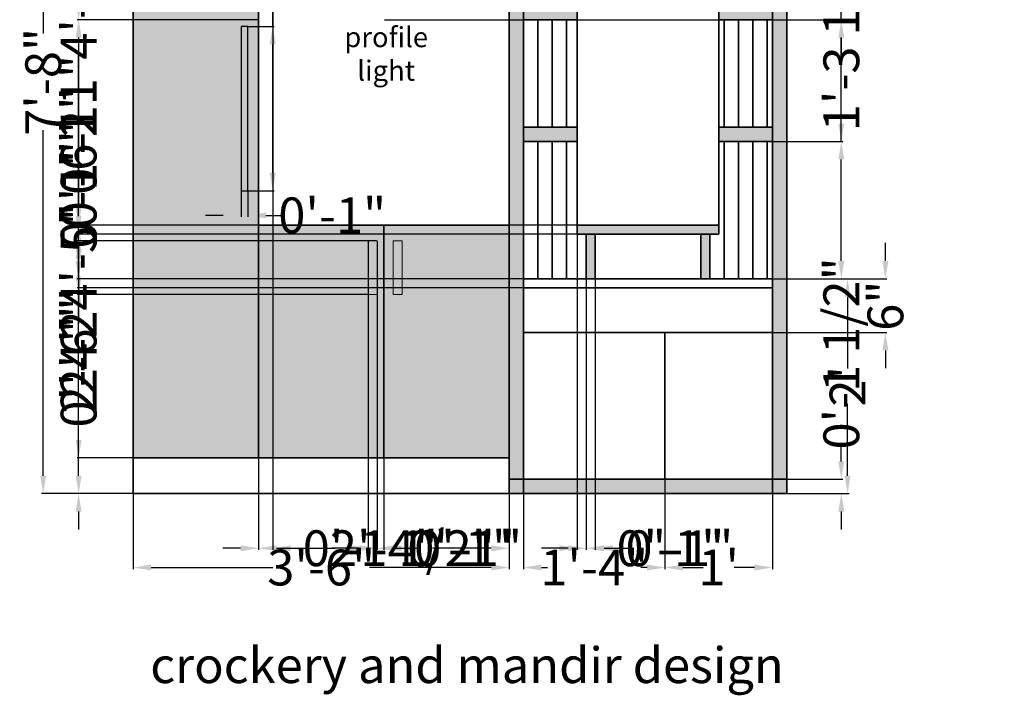
# Model space of a CAD drawing. Units: inches. Extents: x 15 to 125, y 28 to 155.
# Tile 1 of 2: x 15 to 125, y 28 to 104. Entities that reach past the tile are written whole.
import ezdxf

# ---------------------------------------------------------------- set-up
doc = ezdxf.new("R2010")
doc.units = ezdxf.units.IN
doc.header["$MEASUREMENT"] = 0
for name, color, linetype, lineweight in [('A-ANNO-DIMS', 2, 'Continuous', 18), ('A-ANNO-TEXT', 3, 'Continuous', 25), ('A-FURN', 7, 'Continuous', 35), ('A-FURN-HDWR', 8, 'Continuous', 18), ('A-FURN-PATT', 252, 'Continuous', 13)]:
    doc.layers.add(name, color=color, linetype=linetype, lineweight=lineweight)
doc.layers.add('Layer1', color=168, linetype='Continuous')
doc.styles.get("Standard").update_dxf_attribs({"font": 'arial.ttf'})
doc.dimstyles.get("Standard").update_dxf_attribs({"dimtxt": 4, "dimasz": 2, "dimexe": 0.18, "dimexo": 0.0625, "dimgap": 0.09, "dimtad": 0, "dimdec": 0, "dimzin": 0, "dimdsep": 46, "dimlunit": 4, "dimtxsty": 'Standard', "dimcen": 0.09, "dimadec": 0, "dimazin": 0, "dimtfac": 1, "dimtdec": 0, "dimtofl": 0, "dimtmove": 0, "dimatfit": 3, "dimfxl": 1, "dimtolj": 1, "dimtzin": 0, "dimarcsym": 0})

# ---------------------------------------------------------------- blocks, each defined once
blk = doc.blocks.new('*D1')
at = {"layer": 'A-ANNO-DIMS', "color": 0, "lineweight": -2, "transparency": 16777216}
for p, q in [((86.83, 52.41), (86.83, 42.44)), ((98.83, 52.41), (98.83, 42.44)), ((88.83, 42.62), (91.09, 42.62)), ((96.83, 42.62), (94.57, 42.62))]:
    blk.add_line(p, q, dxfattribs=at)
at = {"layer": 'A-ANNO-DIMS', "color": 0, "transparency": 16777216}
for points in [[(88.83, 42.95), (88.83, 42.29), (86.83, 42.62)], [(96.83, 42.95), (96.83, 42.29), (98.83, 42.62)]]:
    blk.add_solid(points, dxfattribs=at)
at = {"layer": 'Defpoints', "color": 0, "transparency": 16777216}
for p in [(86.83, 52.47), (98.83, 52.47), (98.83, 42.62)]:
    blk.add_point(p, dxfattribs=at)
at = {"layer": 'A-ANNO-DIMS', "color": 0, "transparency": 16777216, "insert": (92.83, 42.62), "char_height": 4, "attachment_point": 5}
blk.add_mtext("\\A1;1'", dxfattribs=at)
blk = doc.blocks.new('*D2')
at = {"layer": 'A-ANNO-DIMS', "color": 0, "lineweight": -2, "transparency": 16777216}
for p, q in [((71.03, 52.41), (71.03, 42.44)), ((86.83, 52.41), (86.83, 42.44)), ((73.03, 42.62), (73.71, 42.62)), ((84.83, 42.62), (84.15, 42.62))]:
    blk.add_line(p, q, dxfattribs=at)
at = {"layer": 'A-ANNO-DIMS', "color": 0, "transparency": 16777216}
for points in [[(73.03, 42.95), (73.03, 42.29), (71.03, 42.62)], [(84.83, 42.95), (84.83, 42.29), (86.83, 42.62)]]:
    blk.add_solid(points, dxfattribs=at)
at = {"layer": 'Defpoints', "color": 0, "transparency": 16777216}
for p in [(71.03, 52.47), (86.83, 52.47), (71.03, 42.62)]:
    blk.add_point(p, dxfattribs=at)
at = {"layer": 'A-ANNO-DIMS', "color": 0, "transparency": 16777216, "insert": (78.93, 42.62), "char_height": 4, "attachment_point": 5}
blk.add_mtext('\\A1;1\'-4"', dxfattribs=at)
blk = doc.blocks.new('*D3')
at = {"layer": 'A-ANNO-DIMS', "color": 0, "lineweight": -2, "transparency": 16777216}
for p, q in [((98.89, 74.87), (107.41, 74.87)), ((107.23, 72.87), (107.23, 64.84)), ((107.23, 52.87), (107.23, 60.91)), ((98.89, 50.87), (107.41, 50.87))]:
    blk.add_line(p, q, dxfattribs=at)
at = {"layer": 'A-ANNO-DIMS', "color": 0, "transparency": 16777216}
for points in [[(106.9, 72.87), (107.56, 72.87), (107.23, 74.87)], [(106.9, 52.87), (107.56, 52.87), (107.23, 50.87)]]:
    blk.add_solid(points, dxfattribs=at)
at = {"layer": 'Defpoints', "color": 0, "transparency": 16777216}
for p in [(98.83, 74.87), (107.23, 74.87), (98.83, 50.87)]:
    blk.add_point(p, dxfattribs=at)
at = {"layer": 'A-ANNO-DIMS', "color": 0, "transparency": 16777216, "insert": (107.23, 62.87), "char_height": 4, "attachment_point": 5, "rotation": 90}
blk.add_mtext("\\A1;2'", dxfattribs=at)
blk = doc.blocks.new('*D4')
at = {"layer": 'A-ANNO-DIMS', "color": 0, "lineweight": -2, "transparency": 16777216}
for p, q in [((111.45, 76.87), (111.45, 78.87)), ((98.89, 74.87), (111.63, 74.87)), ((98.89, 68.87), (111.63, 68.87)), ((111.45, 66.87), (111.45, 64.87))]:
    blk.add_line(p, q, dxfattribs=at)
at = {"layer": 'A-ANNO-DIMS', "color": 0, "transparency": 16777216}
for points in [[(111.12, 76.87), (111.79, 76.87), (111.45, 74.87)], [(111.12, 66.87), (111.79, 66.87), (111.45, 68.87)]]:
    blk.add_solid(points, dxfattribs=at)
at = {"layer": 'Defpoints', "color": 0, "transparency": 16777216}
for p in [(98.83, 74.87), (98.83, 68.87), (111.45, 68.87)]:
    blk.add_point(p, dxfattribs=at)
at = {"layer": 'A-ANNO-DIMS', "color": 0, "transparency": 16777216, "insert": (111.45, 71.87), "char_height": 4, "attachment_point": 5, "rotation": 90}
blk.add_mtext('\\A1;6"', dxfattribs=at)
blk = doc.blocks.new('*D8')
at = {"layer": 'A-ANNO-DIMS', "color": 0, "lineweight": -2, "transparency": 16777216}
for p, q in [((27.37, 142.87), (17.19, 142.87)), ((17.37, 140.87), (17.37, 102.26)), ((17.37, 52.87), (17.37, 91.48)), ((27.37, 50.87), (17.19, 50.87))]:
    blk.add_line(p, q, dxfattribs=at)
at = {"layer": 'A-ANNO-DIMS', "color": 0, "transparency": 16777216}
for points in [[(17.04, 140.87), (17.7, 140.87), (17.37, 142.87)], [(17.04, 52.87), (17.7, 52.87), (17.37, 50.87)]]:
    blk.add_solid(points, dxfattribs=at)
at = {"layer": 'Defpoints', "color": 0, "transparency": 16777216}
for p in [(27.43, 142.87), (17.37, 50.87), (27.43, 50.87)]:
    blk.add_point(p, dxfattribs=at)
at = {"layer": 'A-ANNO-DIMS', "color": 0, "transparency": 16777216, "insert": (17.37, 96.87), "char_height": 4, "attachment_point": 5, "rotation": 90}
blk.add_mtext('\\A1;7\'-8"', dxfattribs=at)
blk = doc.blocks.new('*D9')
at = {"layer": 'A-ANNO-DIMS', "color": 0, "lineweight": -2, "transparency": 16777216}
for p, q in [((27.43, 50.81), (27.43, 42.44)), ((69.43, 50.81), (69.43, 42.44)), ((29.43, 42.62), (43.02, 42.62)), ((67.43, 42.62), (53.84, 42.62))]:
    blk.add_line(p, q, dxfattribs=at)
at = {"layer": 'A-ANNO-DIMS', "color": 0, "transparency": 16777216}
for points in [[(29.43, 42.95), (29.43, 42.29), (27.43, 42.62)], [(67.43, 42.95), (67.43, 42.29), (69.43, 42.62)]]:
    blk.add_solid(points, dxfattribs=at)
at = {"layer": 'Defpoints', "color": 0, "transparency": 16777216}
for p in [(27.43, 50.87), (69.43, 50.87), (69.43, 42.62)]:
    blk.add_point(p, dxfattribs=at)
at = {"layer": 'A-ANNO-DIMS', "color": 0, "transparency": 16777216, "insert": (48.43, 42.62), "char_height": 4, "attachment_point": 5}
blk.add_mtext('\\A1;3\'-6"', dxfattribs=at)
blk = doc.blocks.new('SDFDGHJ')
h = blk.add_hatch(color=256)
h.dxf.hatch_style = 1
h.paths.add_polyline_path([(133.35, 265.23), (134.11, 265.23), (134.11, 283.59), (133.35, 283.59)])
at = {"layer": 'Layer1'}
blk.add_lwpolyline([(133.35, 283.59), (133.35, 265.23), (134.11, 265.23), (134.11, 283.59)], close=True, dxfattribs=at)
blk = doc.blocks.new('*D11')
at = {"layer": 'A-ANNO-DIMS', "color": 0, "lineweight": -2, "transparency": 16777216}
for p, q in [((43.01, 103.07), (43.01, 105.07)), ((40.31, 103.07), (43.19, 103.07)), ((43.01, 86.71), (43.01, 101.07)), ((40.31, 84.71), (43.19, 84.71))]:
    blk.add_line(p, q, dxfattribs=at)
at = {"layer": 'A-ANNO-DIMS', "color": 0, "transparency": 16777216}
for points in [[(42.67, 101.07), (43.34, 101.07), (43.01, 103.07)], [(42.67, 86.71), (43.34, 86.71), (43.01, 84.71)]]:
    blk.add_solid(points, dxfattribs=at)
at = {"layer": 'Defpoints', "color": 0, "transparency": 16777216}
for p in [(40.25, 103.07), (43.01, 103.07), (40.25, 84.71)]:
    blk.add_point(p, dxfattribs=at)
at = {"layer": 'A-ANNO-DIMS', "color": 0, "transparency": 16777216, "insert": (43.01, 127.14), "char_height": 4, "attachment_point": 5, "rotation": 90}
blk.add_mtext('\\A1;HANDLE 1\'-6 1/2"', dxfattribs=at)
blk = doc.blocks.new('*D12')
at = {"layer": 'A-ANNO-DIMS', "color": 0, "lineweight": -2, "transparency": 16777216}
for p, q in [((39.49, 84.65), (39.49, 81.78)), ((40.25, 84.65), (40.25, 81.78)), ((37.49, 81.96), (35.49, 81.96)), ((42.25, 81.96), (44.25, 81.96))]:
    blk.add_line(p, q, dxfattribs=at)
at = {"layer": 'A-ANNO-DIMS', "color": 0, "transparency": 16777216}
for points in [[(37.49, 82.29), (37.49, 81.62), (39.49, 81.96)], [(42.25, 82.29), (42.25, 81.62), (40.25, 81.96)]]:
    blk.add_solid(points, dxfattribs=at)
at = {"layer": 'Defpoints', "color": 0, "transparency": 16777216}
for p in [(39.49, 84.71), (40.25, 84.71), (40.25, 81.96)]:
    blk.add_point(p, dxfattribs=at)
at = {"layer": 'A-ANNO-DIMS', "color": 0, "transparency": 16777216, "insert": (49.66, 81.96), "char_height": 4, "attachment_point": 5}
blk.add_mtext('\\A1;0\'-1"', dxfattribs=at)
blk = doc.blocks.new('*D14')
at = {"layer": 'A-ANNO-DIMS', "color": 0, "lineweight": -2, "transparency": 16777216}
for p, q in [((41.43, 142.81), (41.43, 44.59)), ((69.43, 50.81), (69.43, 44.59)), ((43.43, 44.77), (49.99, 44.77)), ((67.43, 44.77), (60.87, 44.77))]:
    blk.add_line(p, q, dxfattribs=at)
at = {"layer": 'A-ANNO-DIMS', "color": 0, "transparency": 16777216}
for points in [[(43.43, 45.1), (43.43, 44.44), (41.43, 44.77)], [(67.43, 45.1), (67.43, 44.44), (69.43, 44.77)]]:
    blk.add_solid(points, dxfattribs=at)
at = {"layer": 'Defpoints', "color": 0, "transparency": 16777216}
for p in [(41.43, 142.87), (69.43, 50.87), (69.43, 44.77)]:
    blk.add_point(p, dxfattribs=at)
at = {"layer": 'A-ANNO-DIMS', "color": 0, "transparency": 16777216, "insert": (55.43, 44.77), "char_height": 4, "attachment_point": 5}
blk.add_mtext('\\A1;2\'-4"', dxfattribs=at)
blk = doc.blocks.new('*D15')
at = {"layer": 'A-ANNO-DIMS', "color": 0, "lineweight": -2, "transparency": 16777216}
for p, q in [((21.33, 56.87), (21.33, 58.87)), ((27.37, 54.87), (21.15, 54.87)), ((27.37, 50.87), (21.15, 50.87)), ((21.33, 48.87), (21.33, 46.87))]:
    blk.add_line(p, q, dxfattribs=at)
at = {"layer": 'A-ANNO-DIMS', "color": 0, "transparency": 16777216}
for points in [[(21, 56.87), (21.66, 56.87), (21.33, 54.87)], [(21, 48.87), (21.66, 48.87), (21.33, 50.87)]]:
    blk.add_solid(points, dxfattribs=at)
at = {"layer": 'Defpoints', "color": 0, "transparency": 16777216}
for p in [(21.33, 54.87), (27.43, 54.87), (27.43, 50.87)]:
    blk.add_point(p, dxfattribs=at)
at = {"layer": 'A-ANNO-DIMS', "color": 0, "transparency": 16777216, "insert": (21.33, 64.28), "char_height": 4, "attachment_point": 5, "rotation": 90}
blk.add_mtext('\\A1;0\'-4"', dxfattribs=at)
blk = doc.blocks.new('*D16')
at = {"layer": 'A-ANNO-DIMS', "color": 0, "lineweight": -2, "transparency": 16777216}
for p, q in [((41.37, 80.87), (21.15, 80.87)), ((21.33, 78.87), (21.33, 71.31)), ((21.33, 52.87), (21.33, 60.43)), ((27.37, 50.87), (21.15, 50.87))]:
    blk.add_line(p, q, dxfattribs=at)
at = {"layer": 'A-ANNO-DIMS', "color": 0, "transparency": 16777216}
for points in [[(21, 78.87), (21.66, 78.87), (21.33, 80.87)], [(21, 52.87), (21.66, 52.87), (21.33, 50.87)]]:
    blk.add_solid(points, dxfattribs=at)
at = {"layer": 'Defpoints', "color": 0, "transparency": 16777216}
for p in [(21.33, 80.87), (41.43, 80.87), (27.43, 50.87)]:
    blk.add_point(p, dxfattribs=at)
at = {"layer": 'A-ANNO-DIMS', "color": 0, "transparency": 16777216, "insert": (21.33, 65.87), "char_height": 4, "attachment_point": 5, "rotation": 90}
blk.add_mtext('\\A1;2\'-6"', dxfattribs=at)
blk = doc.blocks.new('*D17')
at = {"layer": 'A-ANNO-DIMS', "color": 0, "lineweight": -2, "transparency": 16777216}
for p, q in [((41.37, 103.81), (21.15, 103.81)), ((21.33, 101.81), (21.33, 82.83)), ((21.33, 52.87), (21.33, 71.86)), ((27.37, 50.87), (21.15, 50.87))]:
    blk.add_line(p, q, dxfattribs=at)
at = {"layer": 'A-ANNO-DIMS', "color": 0, "transparency": 16777216}
for points in [[(21, 101.81), (21.66, 101.81), (21.33, 103.81)], [(21, 52.87), (21.66, 52.87), (21.33, 50.87)]]:
    blk.add_solid(points, dxfattribs=at)
at = {"layer": 'Defpoints', "color": 0, "transparency": 16777216}
for p in [(21.33, 103.81), (41.43, 103.81), (27.43, 50.87)]:
    blk.add_point(p, dxfattribs=at)
at = {"layer": 'A-ANNO-DIMS', "color": 0, "transparency": 16777216, "insert": (21.33, 77.34), "char_height": 4, "attachment_point": 5, "rotation": 90}
blk.add_mtext('\\A1;4\'-5"', dxfattribs=at)
blk = doc.blocks.new('*D18')
at = {"layer": 'A-ANNO-DIMS', "color": 0, "lineweight": -2, "transparency": 16777216}
for p, q in [((43.03, 105.35), (43.03, 44.59)), ((41.43, 103.75), (41.43, 44.59)), ((39.43, 44.77), (37.43, 44.77)), ((45.03, 44.77), (47.03, 44.77))]:
    blk.add_line(p, q, dxfattribs=at)
at = {"layer": 'A-ANNO-DIMS', "color": 0, "transparency": 16777216}
for points in [[(39.43, 45.1), (39.43, 44.44), (41.43, 44.77)], [(45.03, 45.1), (45.03, 44.44), (43.03, 44.77)]]:
    blk.add_solid(points, dxfattribs=at)
at = {"layer": 'Defpoints', "color": 0, "transparency": 16777216}
for p in [(43.03, 105.41), (41.43, 103.81), (43.03, 44.77)]:
    blk.add_point(p, dxfattribs=at)
at = {"layer": 'A-ANNO-DIMS', "color": 0, "transparency": 16777216, "insert": (57.1, 44.77), "char_height": 4, "attachment_point": 5}
blk.add_mtext('\\A1;0\'-1 1/2"', dxfattribs=at)
blk = doc.blocks.new('*D21')
at = {"layer": 'A-ANNO-DIMS', "color": 0, "lineweight": -2, "transparency": 16777216}
for p, q in [((106.53, 107.41), (106.53, 109.41)), ((56.49, 105.41), (106.71, 105.41)), ((55.49, 103.81), (106.71, 103.81)), ((106.53, 101.81), (106.53, 99.81))]:
    blk.add_line(p, q, dxfattribs=at)
at = {"layer": 'A-ANNO-DIMS', "color": 0, "transparency": 16777216}
for points in [[(106.2, 107.41), (106.86, 107.41), (106.53, 105.41)], [(106.2, 101.81), (106.86, 101.81), (106.53, 103.81)]]:
    blk.add_solid(points, dxfattribs=at)
at = {"layer": 'Defpoints', "color": 0, "transparency": 16777216}
for p in [(56.43, 105.41), (106.53, 105.41), (55.43, 103.81)]:
    blk.add_point(p, dxfattribs=at)
at = {"layer": 'A-ANNO-DIMS', "color": 0, "transparency": 16777216, "insert": (106.53, 119.48), "char_height": 4, "attachment_point": 5, "rotation": 90}
blk.add_mtext('\\A1;0\'-1 1/2"', dxfattribs=at)
blk = doc.blocks.new('*D22')
at = {"layer": 'A-ANNO-DIMS', "color": 0, "lineweight": -2, "transparency": 16777216}
for p, q in [((41.37, 142.87), (21.15, 142.87)), ((21.33, 140.87), (21.33, 128.75)), ((21.33, 105.81), (21.33, 117.94)), ((41.37, 103.81), (21.15, 103.81))]:
    blk.add_line(p, q, dxfattribs=at)
at = {"layer": 'A-ANNO-DIMS', "color": 0, "transparency": 16777216}
for points in [[(21, 140.87), (21.66, 140.87), (21.33, 142.87)], [(21, 105.81), (21.66, 105.81), (21.33, 103.81)]]:
    blk.add_solid(points, dxfattribs=at)
at = {"layer": 'Defpoints', "color": 0, "transparency": 16777216}
for p in [(21.33, 142.87), (41.43, 142.87), (41.43, 103.81)]:
    blk.add_point(p, dxfattribs=at)
at = {"layer": 'A-ANNO-DIMS', "color": 0, "transparency": 16777216, "insert": (21.33, 123.34), "char_height": 4, "attachment_point": 5, "rotation": 90}
blk.add_mtext('\\A1;3\'-3"', dxfattribs=at)
blk = doc.blocks.new('*D23')
at = {"layer": 'A-ANNO-DIMS', "color": 0, "lineweight": -2, "transparency": 16777216}
for p, q in [((41.37, 103.81), (21.15, 103.81)), ((21.33, 101.81), (21.33, 99.12)), ((21.33, 82.87), (21.33, 85.57)), ((41.37, 80.87), (21.15, 80.87))]:
    blk.add_line(p, q, dxfattribs=at)
at = {"layer": 'A-ANNO-DIMS', "color": 0, "transparency": 16777216}
for points in [[(21, 101.81), (21.66, 101.81), (21.33, 103.81)], [(21, 82.87), (21.66, 82.87), (21.33, 80.87)]]:
    blk.add_solid(points, dxfattribs=at)
at = {"layer": 'Defpoints', "color": 0, "transparency": 16777216}
for p in [(21.33, 103.81), (41.43, 103.81), (41.43, 80.87)]:
    blk.add_point(p, dxfattribs=at)
at = {"layer": 'A-ANNO-DIMS', "color": 0, "transparency": 16777216, "insert": (21.33, 92.34), "char_height": 4, "attachment_point": 5, "rotation": 90}
blk.add_mtext('\\A1;1\'-11"', dxfattribs=at)
blk = doc.blocks.new('*D24')
at = {"layer": 'A-ANNO-DIMS', "color": 0, "lineweight": -2, "transparency": 16777216}
for p, q in [((41.37, 80.87), (21.15, 80.87)), ((21.33, 78.87), (21.33, 73.31)), ((21.33, 56.87), (21.33, 62.43)), ((41.37, 54.87), (21.15, 54.87))]:
    blk.add_line(p, q, dxfattribs=at)
at = {"layer": 'A-ANNO-DIMS', "color": 0, "transparency": 16777216}
for points in [[(21, 78.87), (21.66, 78.87), (21.33, 80.87)], [(21, 56.87), (21.66, 56.87), (21.33, 54.87)]]:
    blk.add_solid(points, dxfattribs=at)
at = {"layer": 'Defpoints', "color": 0, "transparency": 16777216}
for p in [(21.33, 80.87), (41.43, 80.87), (41.43, 54.87)]:
    blk.add_point(p, dxfattribs=at)
at = {"layer": 'A-ANNO-DIMS', "color": 0, "transparency": 16777216, "insert": (21.33, 67.87), "char_height": 4, "attachment_point": 5, "rotation": 90}
blk.add_mtext('\\A1;2\'-2"', dxfattribs=at)
blk = doc.blocks.new('*D25')
at = {"layer": 'A-ANNO-DIMS', "color": 0, "lineweight": -2, "transparency": 16777216}
for p, q in [((53.67, 79.06), (53.67, 44.59)), ((54.67, 79.06), (54.67, 44.59)), ((51.67, 44.77), (49.67, 44.77)), ((56.67, 44.77), (58.67, 44.77))]:
    blk.add_line(p, q, dxfattribs=at)
at = {"layer": 'A-ANNO-DIMS', "color": 0, "transparency": 16777216}
for points in [[(51.67, 45.1), (51.67, 44.44), (53.67, 44.77)], [(56.67, 45.1), (56.67, 44.44), (54.67, 44.77)]]:
    blk.add_solid(points, dxfattribs=at)
at = {"layer": 'Defpoints', "color": 0, "transparency": 16777216}
for p in [(53.67, 79.12), (54.67, 79.12), (54.67, 44.77)]:
    blk.add_point(p, dxfattribs=at)
at = {"layer": 'A-ANNO-DIMS', "color": 0, "transparency": 16777216, "insert": (64.07, 44.77), "char_height": 4, "attachment_point": 5}
blk.add_mtext('\\A1;0\'-1"', dxfattribs=at)
blk = doc.blocks.new('*D26')
at = {"layer": 'A-ANNO-DIMS', "color": 0, "lineweight": -2, "transparency": 16777216}
for p, q in [((21.33, 79.12), (21.33, 81.12)), ((53.61, 79.12), (21.15, 79.12)), ((21.33, 75.12), (21.33, 77.12)), ((53.61, 73.12), (21.15, 73.12))]:
    blk.add_line(p, q, dxfattribs=at)
at = {"layer": 'A-ANNO-DIMS', "color": 0, "transparency": 16777216}
for points in [[(21, 77.12), (21.66, 77.12), (21.33, 79.12)], [(21, 75.12), (21.66, 75.12), (21.33, 73.12)]]:
    blk.add_solid(points, dxfattribs=at)
at = {"layer": 'Defpoints', "color": 0, "transparency": 16777216}
for p in [(21.33, 79.12), (53.67, 79.12), (53.67, 73.12)]:
    blk.add_point(p, dxfattribs=at)
at = {"layer": 'A-ANNO-DIMS', "color": 0, "transparency": 16777216, "insert": (21.33, 86.53), "char_height": 4, "attachment_point": 5, "rotation": 90}
blk.add_mtext('\\A1;0\'-6"', dxfattribs=at)
blk = doc.blocks.new('*D27')
at = {"layer": 'A-ANNO-DIMS', "color": 0, "lineweight": -2, "transparency": 16777216}
for p, q in [((21.33, 82.87), (21.33, 84.87)), ((55.37, 80.87), (21.15, 80.87)), ((54.61, 79.12), (21.15, 79.12)), ((21.33, 77.12), (21.33, 75.12))]:
    blk.add_line(p, q, dxfattribs=at)
at = {"layer": 'A-ANNO-DIMS', "color": 0, "transparency": 16777216}
for points in [[(21, 82.87), (21.66, 82.87), (21.33, 80.87)], [(21, 77.12), (21.66, 77.12), (21.33, 79.12)]]:
    blk.add_solid(points, dxfattribs=at)
at = {"layer": 'Defpoints', "color": 0, "transparency": 16777216}
for p in [(21.33, 80.87), (55.43, 80.87), (54.67, 79.12)]:
    blk.add_point(p, dxfattribs=at)
at = {"layer": 'A-ANNO-DIMS', "color": 0, "transparency": 16777216, "insert": (21.33, 90.28), "char_height": 4, "attachment_point": 5, "rotation": 90}
blk.add_mtext('\\A1;0\'-2"', dxfattribs=at)
blk = doc.blocks.new('*D28')
at = {"layer": 'A-ANNO-DIMS', "color": 0, "lineweight": -2, "transparency": 16777216}
for p, q in [((55.43, 80.81), (55.43, 44.59)), ((54.67, 79.06), (54.67, 44.59)), ((52.67, 44.77), (50.67, 44.77)), ((57.43, 44.77), (59.43, 44.77))]:
    blk.add_line(p, q, dxfattribs=at)
at = {"layer": 'A-ANNO-DIMS', "color": 0, "transparency": 16777216}
for points in [[(52.67, 45.1), (52.67, 44.44), (54.67, 44.77)], [(57.43, 45.1), (57.43, 44.44), (55.43, 44.77)]]:
    blk.add_solid(points, dxfattribs=at)
at = {"layer": 'Defpoints', "color": 0, "transparency": 16777216}
for p in [(55.43, 80.87), (54.67, 79.12), (55.43, 44.77)]:
    blk.add_point(p, dxfattribs=at)
at = {"layer": 'A-ANNO-DIMS', "color": 0, "transparency": 16777216, "insert": (64.84, 44.77), "char_height": 4, "attachment_point": 5}
blk.add_mtext('\\A1;0\'-1"', dxfattribs=at)
blk = doc.blocks.new('*D29')
at = {"layer": 'A-ANNO-DIMS', "color": 0, "lineweight": -2, "transparency": 16777216}
for p, q in [((96.83, 148.97), (94.83, 148.97)), ((98.83, 74.93), (98.83, 149.15)), ((100.43, 50.93), (100.43, 149.15)), ((102.43, 148.97), (104.43, 148.97))]:
    blk.add_line(p, q, dxfattribs=at)
at = {"layer": 'A-ANNO-DIMS', "color": 0, "transparency": 16777216}
for points in [[(96.83, 149.3), (96.83, 148.64), (98.83, 148.97)], [(102.43, 149.3), (102.43, 148.64), (100.43, 148.97)]]:
    blk.add_solid(points, dxfattribs=at)
at = {"layer": 'Defpoints', "color": 0, "transparency": 16777216}
for p in [(100.43, 148.97), (98.83, 74.87), (100.43, 50.87)]:
    blk.add_point(p, dxfattribs=at)
at = {"layer": 'A-ANNO-DIMS', "color": 0, "transparency": 16777216, "insert": (114.5, 148.97), "char_height": 4, "attachment_point": 5}
blk.add_mtext('\\A1;0\'-1 1/2"', dxfattribs=at)
blk = doc.blocks.new('*D33')
at = {"layer": 'A-ANNO-DIMS', "color": 0, "lineweight": -2, "transparency": 16777216}
for p, q in [((76.97, 130.87), (21.15, 130.87)), ((21.33, 128.87), (21.33, 110.86)), ((21.33, 81.87), (21.33, 99.88)), ((76.97, 79.87), (21.15, 79.87))]:
    blk.add_line(p, q, dxfattribs=at)
at = {"layer": 'A-ANNO-DIMS', "color": 0, "transparency": 16777216}
for points in [[(21, 128.87), (21.66, 128.87), (21.33, 130.87)], [(21, 81.87), (21.66, 81.87), (21.33, 79.87)]]:
    blk.add_solid(points, dxfattribs=at)
at = {"layer": 'Defpoints', "color": 0, "transparency": 16777216}
for p in [(21.33, 130.87), (77.03, 130.87), (77.03, 79.87)]:
    blk.add_point(p, dxfattribs=at)
at = {"layer": 'A-ANNO-DIMS', "color": 0, "transparency": 16777216, "insert": (21.33, 105.37), "char_height": 4, "attachment_point": 5, "rotation": 90}
blk.add_mtext('\\A1;4\'-3"', dxfattribs=at)
blk = doc.blocks.new('*D34')
at = {"layer": 'A-ANNO-DIMS', "color": 0, "lineweight": -2, "transparency": 16777216}
for p, q in [((106.53, 90.21), (106.53, 92.21)), ((98.89, 90.21), (106.71, 90.21)), ((106.53, 76.87), (106.53, 88.21)), ((98.89, 74.87), (106.71, 74.87))]:
    blk.add_line(p, q, dxfattribs=at)
at = {"layer": 'A-ANNO-DIMS', "color": 0, "transparency": 16777216}
for points in [[(106.2, 88.21), (106.86, 88.21), (106.53, 90.21)], [(106.2, 76.87), (106.86, 76.87), (106.53, 74.87)]]:
    blk.add_solid(points, dxfattribs=at)
at = {"layer": 'Defpoints', "color": 0, "transparency": 16777216}
for p in [(98.83, 90.21), (106.53, 90.21), (98.83, 74.87)]:
    blk.add_point(p, dxfattribs=at)
at = {"layer": 'A-ANNO-DIMS', "color": 0, "transparency": 16777216, "insert": (106.53, 102.09), "char_height": 4, "attachment_point": 5, "rotation": 90}
blk.add_mtext('\\A1;1\'-3 1/2"', dxfattribs=at)
blk = doc.blocks.new('*D35')
at = {"layer": 'A-ANNO-DIMS', "color": 0, "lineweight": -2, "transparency": 16777216}
for p, q in [((106.53, 103.81), (106.53, 105.81)), ((98.89, 103.81), (106.71, 103.81)), ((106.53, 92.21), (106.53, 101.81)), ((98.89, 90.21), (106.71, 90.21))]:
    blk.add_line(p, q, dxfattribs=at)
at = {"layer": 'A-ANNO-DIMS', "color": 0, "transparency": 16777216}
for points in [[(106.2, 101.81), (106.86, 101.81), (106.53, 103.81)], [(106.2, 92.21), (106.86, 92.21), (106.53, 90.21)]]:
    blk.add_solid(points, dxfattribs=at)
at = {"layer": 'Defpoints', "color": 0, "transparency": 16777216}
for p in [(98.83, 103.81), (106.53, 103.81), (98.83, 90.21)]:
    blk.add_point(p, dxfattribs=at)
at = {"layer": 'A-ANNO-DIMS', "color": 0, "transparency": 16777216, "insert": (106.53, 115.69), "char_height": 4, "attachment_point": 5, "rotation": 90}
blk.add_mtext('\\A1;1\'-1 1/2"', dxfattribs=at)
blk = doc.blocks.new('*D36')
at = {"layer": 'A-ANNO-DIMS', "color": 0, "lineweight": -2, "transparency": 16777216}
for p, q in [((106.53, 117.41), (106.53, 119.41)), ((98.89, 117.41), (106.71, 117.41)), ((106.53, 105.81), (106.53, 115.41)), ((98.89, 103.81), (106.71, 103.81))]:
    blk.add_line(p, q, dxfattribs=at)
at = {"layer": 'A-ANNO-DIMS', "color": 0, "transparency": 16777216}
for points in [[(106.2, 115.41), (106.86, 115.41), (106.53, 117.41)], [(106.2, 105.81), (106.86, 105.81), (106.53, 103.81)]]:
    blk.add_solid(points, dxfattribs=at)
at = {"layer": 'Defpoints', "color": 0, "transparency": 16777216}
for p in [(98.83, 117.41), (106.53, 117.41), (98.83, 103.81)]:
    blk.add_point(p, dxfattribs=at)
at = {"layer": 'A-ANNO-DIMS', "color": 0, "transparency": 16777216, "insert": (106.53, 129.29), "char_height": 4, "attachment_point": 5, "rotation": 90}
blk.add_mtext('\\A1;1\'-1 1/2"', dxfattribs=at)
blk = doc.blocks.new('*D39')
at = {"layer": 'A-ANNO-DIMS', "color": 0, "lineweight": -2, "transparency": 16777216}
for p, q in [((77.03, 79.81), (77.03, 44.59)), ((78.03, 79.81), (78.03, 44.59)), ((75.03, 44.77), (73.03, 44.77)), ((80.03, 44.77), (82.03, 44.77))]:
    blk.add_line(p, q, dxfattribs=at)
at = {"layer": 'A-ANNO-DIMS', "color": 0, "transparency": 16777216}
for points in [[(75.03, 45.1), (75.03, 44.44), (77.03, 44.77)], [(80.03, 45.1), (80.03, 44.44), (78.03, 44.77)]]:
    blk.add_solid(points, dxfattribs=at)
at = {"layer": 'Defpoints', "color": 0, "transparency": 16777216}
for p in [(77.03, 79.87), (78.03, 79.87), (78.03, 44.77)]:
    blk.add_point(p, dxfattribs=at)
at = {"layer": 'A-ANNO-DIMS', "color": 0, "transparency": 16777216, "insert": (87.44, 44.77), "char_height": 4, "attachment_point": 5}
blk.add_mtext('\\A1;0\'-1"', dxfattribs=at)
blk = doc.blocks.new('*D40')
at = {"layer": 'A-ANNO-DIMS', "color": 0, "lineweight": -2, "transparency": 16777216}
for p, q in [((78.03, 79.81), (78.03, 44.59)), ((79.03, 79.81), (79.03, 44.59)), ((76.03, 44.77), (74.03, 44.77)), ((81.03, 44.77), (83.03, 44.77))]:
    blk.add_line(p, q, dxfattribs=at)
at = {"layer": 'A-ANNO-DIMS', "color": 0, "transparency": 16777216}
for points in [[(76.03, 45.1), (76.03, 44.44), (78.03, 44.77)], [(81.03, 45.1), (81.03, 44.44), (79.03, 44.77)]]:
    blk.add_solid(points, dxfattribs=at)
at = {"layer": 'Defpoints', "color": 0, "transparency": 16777216}
for p in [(78.03, 79.87), (79.03, 79.87), (79.03, 44.77)]:
    blk.add_point(p, dxfattribs=at)
at = {"layer": 'A-ANNO-DIMS', "color": 0, "transparency": 16777216, "insert": (88.44, 44.77), "char_height": 4, "attachment_point": 5}
blk.add_mtext('\\A1;0\'-1"', dxfattribs=at)
blk = doc.blocks.new('*D41')
at = {"layer": 'A-ANNO-DIMS', "color": 0, "lineweight": -2, "transparency": 16777216}
for p, q in [((21.33, 82.87), (21.33, 84.87)), ((76.97, 80.87), (21.15, 80.87)), ((76.97, 79.87), (21.15, 79.87)), ((21.33, 77.87), (21.33, 75.87))]:
    blk.add_line(p, q, dxfattribs=at)
at = {"layer": 'A-ANNO-DIMS', "color": 0, "transparency": 16777216}
for points in [[(21, 82.87), (21.66, 82.87), (21.33, 80.87)], [(21, 77.87), (21.66, 77.87), (21.33, 79.87)]]:
    blk.add_solid(points, dxfattribs=at)
at = {"layer": 'Defpoints', "color": 0, "transparency": 16777216}
for p in [(21.33, 80.87), (77.03, 80.87), (77.03, 79.87)]:
    blk.add_point(p, dxfattribs=at)
at = {"layer": 'A-ANNO-DIMS', "color": 0, "transparency": 16777216, "insert": (21.33, 90.28), "char_height": 4, "attachment_point": 5, "rotation": 90}
blk.add_mtext('\\A1;0\'-1"', dxfattribs=at)
blk = doc.blocks.new('*D42')
at = {"layer": 'A-ANNO-DIMS', "color": 0, "lineweight": -2, "transparency": 16777216}
for p, q in [((21.33, 76.87), (21.33, 78.87)), ((70.97, 74.87), (21.15, 74.87)), ((70.97, 73.87), (21.15, 73.87)), ((21.33, 71.87), (21.33, 69.87))]:
    blk.add_line(p, q, dxfattribs=at)
at = {"layer": 'A-ANNO-DIMS', "color": 0, "transparency": 16777216}
for points in [[(21, 76.87), (21.66, 76.87), (21.33, 74.87)], [(21, 71.87), (21.66, 71.87), (21.33, 73.87)]]:
    blk.add_solid(points, dxfattribs=at)
at = {"layer": 'Defpoints', "color": 0, "transparency": 16777216}
for p in [(21.33, 74.87), (71.03, 74.87), (71.03, 73.87)]:
    blk.add_point(p, dxfattribs=at)
at = {"layer": 'A-ANNO-DIMS', "color": 0, "transparency": 16777216, "insert": (21.33, 84.28), "char_height": 4, "attachment_point": 5, "rotation": 90}
blk.add_mtext('\\A1;0\'-1"', dxfattribs=at)
blk = doc.blocks.new('*D43')
at = {"layer": 'A-ANNO-DIMS', "color": 0, "lineweight": -2, "transparency": 16777216}
for p, q in [((106.53, 54.47), (106.53, 56.47)), ((100.49, 52.47), (106.71, 52.47)), ((100.49, 50.87), (106.71, 50.87)), ((106.53, 48.87), (106.53, 46.87))]:
    blk.add_line(p, q, dxfattribs=at)
at = {"layer": 'A-ANNO-DIMS', "color": 0, "transparency": 16777216}
for points in [[(106.2, 54.47), (106.86, 54.47), (106.53, 52.47)], [(106.2, 48.87), (106.86, 48.87), (106.53, 50.87)]]:
    blk.add_solid(points, dxfattribs=at)
at = {"layer": 'Defpoints', "color": 0, "transparency": 16777216}
for p in [(100.43, 52.47), (106.53, 52.47), (100.43, 50.87)]:
    blk.add_point(p, dxfattribs=at)
at = {"layer": 'A-ANNO-DIMS', "color": 0, "transparency": 16777216, "insert": (106.53, 66.54), "char_height": 4, "attachment_point": 5, "rotation": 90}
blk.add_mtext('\\A1;0\'-1 1/2"', dxfattribs=at)

msp = doc.modelspace()

# ---------------------------------------------------------------- hatches: boundary and pattern name
at = {"layer": 'A-FURN-PATT'}
h = msp.add_hatch(color=256, dxfattribs=at)
h.dxf.hatch_style = 1
h.paths.add_polyline_path([(55.43, 80.87), (41.43, 80.87), (41.43, 54.87), (55.43, 54.87)])
h.paths.add_polyline_path([(69.43, 80.87), (55.43, 80.87), (55.43, 54.87), (69.43, 54.87)])
h.paths.add_polyline_path([(41.43, 80.87), (41.43, 142.87), (27.43, 142.87), (27.43, 54.87), (41.43, 54.87)])
h = msp.add_hatch(color=256, dxfattribs=at)
h.dxf.hatch_style = 1
h.paths.add_polyline_path([(71.03, 141.27), (98.83, 141.27), (98.83, 50.87), (100.43, 50.87), (100.43, 142.87), (69.43, 142.87), (69.43, 50.87), (71.03, 50.87)])
h = msp.add_hatch(color=256, dxfattribs=at)
h.dxf.hatch_style = 1
h.paths.add_polyline_path([(77.03, 119.01), (71.03, 119.01), (71.03, 117.41), (77.03, 117.41)])
h.paths.add_polyline_path([(98.83, 119.01), (92.83, 119.01), (92.83, 117.41), (98.83, 117.41)])
h.paths.add_polyline_path([(98.83, 105.41), (92.83, 105.41), (92.83, 103.81), (98.83, 103.81)])
h.paths.add_polyline_path([(77.03, 105.41), (71.03, 105.41), (71.03, 103.81), (77.03, 103.81)])
h.paths.add_polyline_path([(98.83, 91.81), (92.83, 91.81), (92.83, 90.21), (98.83, 90.21)])
h.paths.add_polyline_path([(77.03, 91.81), (71.03, 91.81), (71.03, 90.21), (77.03, 90.21)])
h = msp.add_hatch(color=256, dxfattribs=at)
h.dxf.hatch_style = 1
h.paths.add_polyline_path([(92.83, 80.87), (77.03, 80.87), (77.03, 79.87), (92.83, 79.87)])
h.paths.add_polyline_path([(91.83, 79.87), (90.83, 79.87), (90.83, 74.87), (91.83, 74.87)])
h.paths.add_polyline_path([(79.03, 79.87), (78.03, 79.87), (78.03, 74.87), (79.03, 74.87)])
h = msp.add_hatch(color=256, dxfattribs=at)
h.dxf.hatch_style = 1
h.paths.add_polyline_path([(53.67, 73.12), (54.67, 73.12), (54.67, 79.12), (53.67, 79.12)])
h = msp.add_hatch(color=256, dxfattribs=at)
h.dxf.hatch_style = 1
h.paths.add_polyline_path([(56.46, 73.12), (57.46, 73.12), (57.46, 79.12), (56.46, 79.12)])
h = msp.add_hatch(color=256, dxfattribs=at)
h.dxf.hatch_style = 1
h.paths.add_polyline_path([(98.83, 50.87), (98.83, 52.47), (71.03, 52.47), (71.03, 50.87)])

# ---------------------------------------------------------------- linework, layer by layer
at = {"layer": 'A-FURN'}
for p, q in [((27.43, 142.87), (27.43, 50.87)), ((41.43, 142.87), (41.43, 54.87)), ((77.03, 130.87), (77.03, 80.87)), ((92.83, 130.87), (92.83, 80.87)), ((77.03, 103.81), (71.03, 103.81)), ((72.63, 91.81), (72.63, 103.81)), ((74.23, 91.81), (74.23, 103.81)), ((75.83, 91.81), (75.83, 103.81)), ((98.83, 103.81), (92.83, 103.81)), ((93.43, 91.81), (93.43, 103.81)), ((95.03, 91.81), (95.03, 103.81)), ((96.63, 91.81), (96.63, 103.81)), ((98.23, 91.81), (98.23, 103.81)), ((71.03, 91.81), (77.03, 91.81)), ((92.83, 91.81), (98.83, 91.81)), ((77.03, 90.21), (71.03, 90.21)), ((72.63, 74.87), (72.63, 90.21)), ((74.23, 74.87), (74.23, 90.21)), ((75.83, 74.87), (75.83, 90.21)), ((98.83, 90.21), (92.83, 90.21)), ((93.43, 74.87), (93.43, 90.21)), ((95.03, 74.87), (95.03, 90.21)), ((96.63, 74.87), (96.63, 90.21)), ((98.23, 74.87), (98.23, 90.21)), ((41.43, 80.87), (69.43, 80.87)), ((55.43, 80.87), (55.43, 54.87)), ((92.83, 80.87), (77.03, 80.87)), ((77.03, 80.87), (77.03, 79.87)), ((92.83, 80.87), (92.83, 79.87)), ((92.83, 79.87), (77.03, 79.87)), ((78.03, 79.87), (78.03, 74.87)), ((79.03, 79.87), (79.03, 74.87)), ((79.03, 74.87), (79.03, 79.87)), ((90.83, 79.87), (90.83, 74.87)), ((91.83, 79.87), (91.83, 74.87)), ((91.83, 74.87), (91.83, 79.87)), ((98.83, 74.87), (71.03, 74.87)), ((98.83, 73.87), (71.03, 73.87)), ((98.83, 68.87), (71.03, 68.87)), ((86.83, 68.87), (86.83, 52.47)), ((69.43, 54.87), (27.43, 54.87)), ((100.43, 52.47), (69.43, 52.47)), ((27.43, 50.87), (69.43, 50.87))]:
    msp.add_line(p, q, dxfattribs=at)
msp.add_lwpolyline([(100.43, 142.87), (100.43, 50.87), (69.43, 50.87), (69.43, 142.87)], close=True, dxfattribs=at)
msp.add_lwpolyline([(98.83, 50.87), (98.83, 141.27), (71.03, 141.27), (71.03, 50.87)], dxfattribs=at)
at = {"layer": 'A-FURN-HDWR'}
for points in [[(53.67, 73.12), (54.67, 73.12), (54.67, 79.12), (53.67, 79.12)], [(56.46, 73.12), (57.46, 73.12), (57.46, 79.12), (56.46, 79.12)]]:
    msp.add_lwpolyline(points, close=True, dxfattribs=at)

# ---------------------------------------------------------------- block references
msp.add_blockref('SDFDGHJ', (-93.86, -180.52), dxfattribs=at)

# ---------------------------------------------------------------- texts
at = {"layer": 'A-ANNO-TEXT', "attachment_point": 1}
for s, width, gutter_width, insert, char_height in [('\\pxqc;profile light', 15.2347, 11.22, (48.07, 102.99), 2.2448), ('\\pxqc;crockery and mandir design', 79.1063, 20, (25.16, 33.71), 4)]:
    msp.add_mtext_dynamic_manual_height_columns(s, width=width, gutter_width=gutter_width, heights=[0], dxfattribs=dict(at, insert=insert, char_height=char_height))

# ---------------------------------------------------------------- dimensions: what is measured, and where the dimension line sits
at = {"layer": 'A-ANNO-DIMS'}
for base, p1, p2, override, picture, middle in [((100.43, 148.97), (98.83, 74.87), (100.43, 50.87), {"dimdec": 1, "dimlfac": 1, "dimrnd": 0, "dimzin": 1, "dimdsep": 46, "dimlunit": 4, "dimfrac": 2}, '*D29', (114.5, 148.97)), ((69.43, 44.77), (41.43, 142.87), (69.43, 50.87), {"dimdec": 1, "dimlfac": 1, "dimrnd": 0, "dimzin": 1, "dimdsep": 46, "dimlunit": 4, "dimfrac": 2}, '*D14', (55.43, 44.77)), ((43.03, 44.77), (41.43, 103.81), (43.03, 105.41), {"dimdec": 1, "dimlfac": 1, "dimrnd": 0, "dimzin": 1, "dimdsep": 46, "dimlunit": 4, "dimfrac": 2}, '*D18', (57.1, 44.77)), ((40.25, 81.96), (39.49, 84.71), (40.25, 84.71), {"dimdec": 1, "dimrnd": 0, "dimzin": 1, "dimlunit": 4, "dimfrac": 2}, '*D12', (49.66, 81.96)), ((55.43, 44.77), (54.67, 79.12), (55.43, 80.87), {"dimdec": 1, "dimlfac": 1, "dimrnd": 0, "dimzin": 1, "dimdsep": 46, "dimlunit": 4, "dimfrac": 2}, '*D28', (64.84, 44.77)), ((78.03, 44.77), (77.03, 79.87), (78.03, 79.87), {"dimdec": 1, "dimlfac": 1, "dimrnd": 0, "dimzin": 1, "dimdsep": 46, "dimlunit": 4, "dimfrac": 2}, '*D39', (87.44, 44.77)), ((79.03, 44.77), (78.03, 79.87), (79.03, 79.87), {"dimdec": 1, "dimlfac": 1, "dimrnd": 0, "dimzin": 1, "dimdsep": 46, "dimlunit": 4, "dimfrac": 2}, '*D40', (88.44, 44.77)), ((54.67, 44.77), (53.67, 79.12), (54.67, 79.12), {"dimdec": 1, "dimlfac": 1, "dimrnd": 0, "dimzin": 1, "dimdsep": 46, "dimlunit": 4, "dimfrac": 2}, '*D25', (64.07, 44.77)), ((71.03, 42.62), (86.83, 52.47), (71.03, 52.47), {"dimclrd": 0, "dimclre": 0, "dimclrt": 0}, '*D2', (78.93, 42.62)), ((98.83, 42.62), (86.83, 52.47), (98.83, 52.47), {"dimclrd": 0, "dimclre": 0, "dimclrt": 0}, '*D1', (92.83, 42.62)), ((69.43, 42.62), (27.43, 50.87), (69.43, 50.87), {"dimclrd": 0, "dimclre": 0, "dimclrt": 0}, '*D9', (48.43, 42.62))]:
    dim = msp.add_linear_dim(base=base, p1=p1, p2=p2, dimstyle='Standard', override=override, dxfattribs=at)
    dim.commit()
    dim.dimension.update_dxf_attribs({"geometry": picture, "text_midpoint": middle})
dim = msp.add_linear_dim(base=(43.01, 103.07), p1=(40.25, 84.71), p2=(40.25, 103.07), angle=90, text='HANDLE <>', dimstyle='Standard', override={"dimdec": 1, "dimrnd": 0, "dimzin": 1, "dimlunit": 4, "dimfrac": 2}, dxfattribs=at)
dim.commit()
dim.dimension.update_dxf_attribs({"geometry": '*D11', "text_midpoint": (43.01, 127.14)})
for base, p1, p2, override, picture, middle in [((17.37, 50.87), (27.43, 142.87), (27.43, 50.87), {"dimclrd": 0, "dimclre": 0, "dimclrt": 0}, '*D8', (17.37, 96.87)), ((21.33, 142.87), (41.43, 103.81), (41.43, 142.87), {"dimdec": 1, "dimlfac": 1, "dimrnd": 0, "dimzin": 1, "dimdsep": 46, "dimlunit": 4, "dimfrac": 2}, '*D22', (21.33, 123.34)), ((106.53, 117.41), (98.83, 103.81), (98.83, 117.41), {"dimdec": 1, "dimlfac": 1, "dimrnd": 0, "dimzin": 1, "dimdsep": 46, "dimlunit": 4, "dimfrac": 2}, '*D36', (106.53, 129.29)), ((21.33, 130.87), (77.03, 79.87), (77.03, 130.87), {"dimdec": 1, "dimlfac": 1, "dimrnd": 0, "dimzin": 1, "dimdsep": 46, "dimlunit": 4, "dimfrac": 2}, '*D33', (21.33, 105.37)), ((106.53, 105.41), (55.43, 103.81), (56.43, 105.41), {"dimdec": 1, "dimlfac": 1, "dimrnd": 0, "dimzin": 1, "dimdsep": 46, "dimlunit": 4, "dimfrac": 2}, '*D21', (106.53, 119.48)), ((106.53, 103.81), (98.83, 90.21), (98.83, 103.81), {"dimdec": 1, "dimlfac": 1, "dimrnd": 0, "dimzin": 1, "dimdsep": 46, "dimlunit": 4, "dimfrac": 2}, '*D35', (106.53, 115.69)), ((106.53, 90.21), (98.83, 74.87), (98.83, 90.21), {"dimdec": 1, "dimlfac": 1, "dimrnd": 0, "dimzin": 1, "dimdsep": 46, "dimlunit": 4, "dimfrac": 2}, '*D34', (106.53, 102.09)), ((21.33, 103.81), (27.43, 50.87), (41.43, 103.81), {"dimdec": 1, "dimlfac": 1, "dimrnd": 0, "dimzin": 1, "dimdsep": 46, "dimlunit": 4, "dimfrac": 2}, '*D17', (21.33, 77.34)), ((21.33, 103.81), (41.43, 80.87), (41.43, 103.81), {"dimdec": 1, "dimlfac": 1, "dimrnd": 0, "dimzin": 1, "dimdsep": 46, "dimlunit": 4, "dimfrac": 2}, '*D23', (21.33, 92.34)), ((21.3299, 80.8712), (54.6684, 79.1189), (55.4299, 80.8712), {"dimdec": 1, "dimlfac": 1, "dimrnd": 0, "dimzin": 1, "dimdsep": 46, "dimlunit": 4, "dimfrac": 2}, '*D27', (21.3299, 90.2777)), ((21.33, 80.87), (77.03, 79.87), (77.03, 80.87), {"dimdec": 1, "dimlfac": 1, "dimrnd": 0, "dimzin": 1, "dimdsep": 46, "dimlunit": 4, "dimfrac": 2}, '*D41', (21.33, 90.28)), ((21.33, 79.12), (53.67, 73.12), (53.67, 79.12), {"dimdec": 1, "dimlfac": 1, "dimrnd": 0, "dimzin": 1, "dimdsep": 46, "dimlunit": 4, "dimfrac": 2}, '*D26', (21.33, 86.53)), ((21.33, 74.87), (71.03, 73.87), (71.03, 74.87), {"dimdec": 1, "dimlfac": 1, "dimrnd": 0, "dimzin": 1, "dimdsep": 46, "dimlunit": 4, "dimfrac": 2}, '*D42', (21.33, 84.28)), ((21.33, 80.87), (27.43, 50.87), (41.43, 80.87), {"dimdec": 1, "dimlfac": 1, "dimrnd": 0, "dimzin": 1, "dimdsep": 46, "dimlunit": 4, "dimfrac": 2}, '*D16', (21.33, 65.87)), ((21.33, 80.87), (41.43, 54.87), (41.43, 80.87), {"dimdec": 1, "dimlfac": 1, "dimrnd": 0, "dimzin": 1, "dimdsep": 46, "dimlunit": 4, "dimfrac": 2}, '*D24', (21.33, 67.87)), ((111.45, 68.87), (98.83, 74.87), (98.83, 68.87), {"dimclrd": 0, "dimclre": 0, "dimclrt": 0}, '*D4', (111.45, 71.87)), ((106.53, 52.47), (100.43, 50.87), (100.43, 52.47), {"dimdec": 1, "dimlfac": 1, "dimrnd": 0, "dimzin": 1, "dimdsep": 46, "dimlunit": 4, "dimfrac": 2}, '*D43', (106.53, 66.54)), ((107.23, 74.87), (98.83, 50.87), (98.83, 74.87), {"dimclrd": 0, "dimclre": 0, "dimclrt": 0}, '*D3', (107.23, 62.87)), ((21.33, 54.87), (27.43, 50.87), (27.43, 54.87), {"dimdec": 1, "dimlfac": 1, "dimrnd": 0, "dimzin": 1, "dimdsep": 46, "dimlunit": 4, "dimfrac": 2}, '*D15', (21.33, 64.28))]:
    dim = msp.add_linear_dim(base=base, p1=p1, p2=p2, angle=90, dimstyle='Standard', override=override, dxfattribs=at)
    dim.commit()
    dim.dimension.update_dxf_attribs({"geometry": picture, "text_midpoint": middle})

doc.saveas('drawing.dxf')
